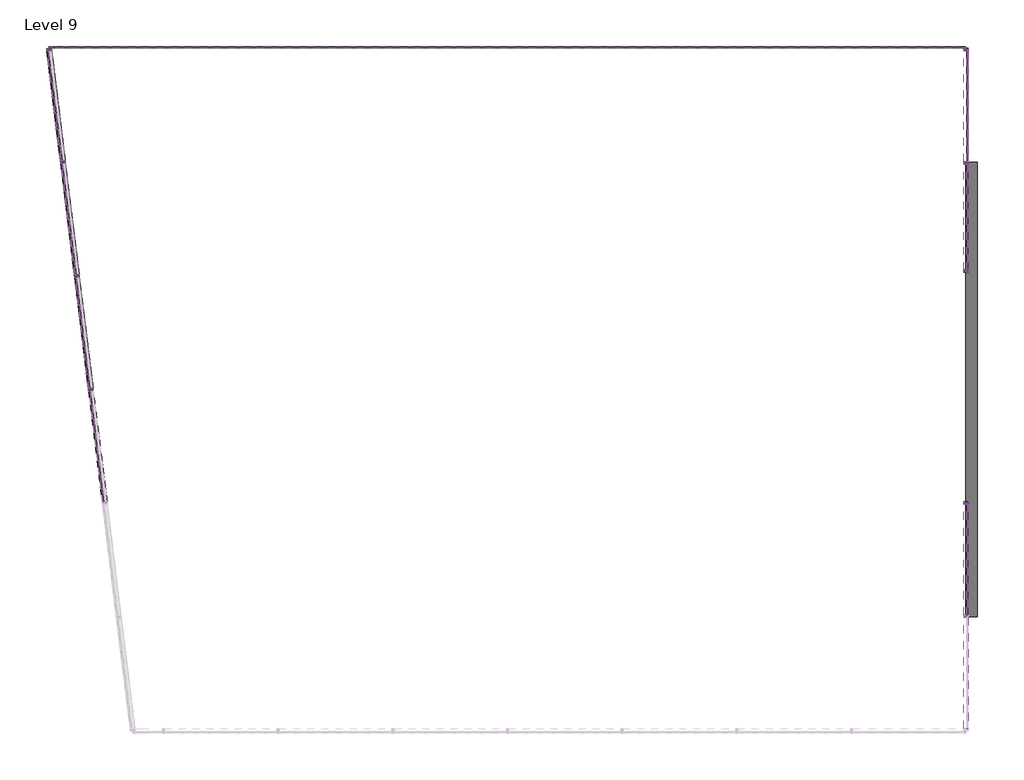
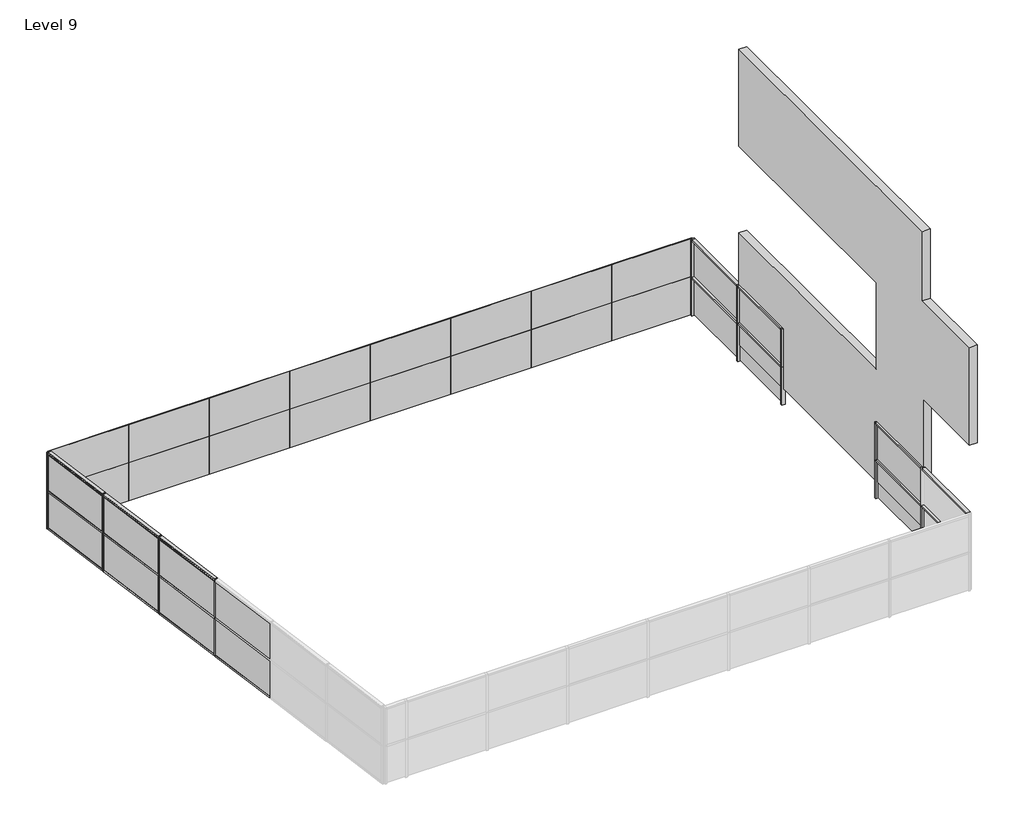
# One storey, part 2 of 2: 49 members, 38 plates, 1 proxy.
"""IFC4 building model written with IfcOpenShell, lengths in millimetres."""

from ifc_helpers import new_model, si_unit, origin, place, context, project, spatial, transform, mapped, element, save
from components import generic_models_4_generic_models_1_d225a6a7, member_71c27fd2, member_daa7a266, member_82905deb, member_19d0a4ec, member_8cef0660, member_db480205, member_4491d118, member_46bdb8c2, member_1b94d493, system_panel_glazed_1e57f9bb, system_panel_glazed_37f15d2e, system_panel_glazed_3620f98e, system_panel_glazed_e46d4b42, system_panel_glazed_2a6c68b7, system_panel_glazed_7fb1fc2b, system_panel_glazed_d483336f

model = new_model("IFC4")

# Units and contexts
model_context = context("Model", 3, world=origin())
ifc_project = project(units=[si_unit("LENGTHUNIT", "METRE", prefix="MILLI")], contexts=[model_context])

# Site, building, storey
site = spatial("IfcSite", under=ifc_project)
building = spatial("IfcBuilding", under=site)
storey = spatial("IfcBuildingStorey", under=building, Name="Level 9", Elevation=24384.0)

# Proxy
placement = place(None, origin())
generic_models_4_generic_models_1_shape = generic_models_4_generic_models_1_d225a6a7(model_context)
element("IfcBuildingElementProxy", 1, Name="Generic Models 4 : Generic Models 1", ObjectType="Generic Models 4 : Generic Models 1", at=placement, inside=storey, context=model_context, shape_type="MappedRepresentation", body=[
    mapped(generic_models_4_generic_models_1_shape, transform((0.0, 0.0, 27943.2641305), x_axis=(1.0, 0.0, 0.0), y_axis=(0.0, 1.0, 0.0), z_axis=(0.0, 0.0, 1.0))),
])

# Members
member_shape = member_71c27fd2(model_context)
element("IfcMember", 2, ObjectType="Rectangular Mullion : 2.5\" x 5\" rectangular", at=placement, inside=storey, context=model_context, shape_type="MappedRepresentation", body=[
    mapped(member_shape, transform((-10473.7456604, 11109.5209701, 24384.0), x_axis=(0.0, 0.0, -1.0), y_axis=(-0.9925461516413222, -0.12186934340514603, 0.0), z_axis=(-0.12186934340514603, 0.9925461516413222, 0.0))),
])
member_2_shape = member_daa7a266(model_context)
element("IfcMember", 3, ObjectType="Rectangular Mullion : 2.5\" x 5\" rectangular", at=placement, inside=storey, context=model_context, shape_type="MappedRepresentation", body=[
    mapped(member_2_shape, transform((-10113.8959567, 8178.7803212, 27432.0), x_axis=(0.0, 0.0, 1.0), y_axis=(-0.9925461516413222, -0.12186934340514613, 0.0), z_axis=(0.12186934340514613, -0.9925461516413222, 0.0))),
])
element("IfcMember", 4, ObjectType="Rectangular Mullion : 2.5\" x 5\" rectangular", at=placement, inside=storey, context=model_context, shape_type="MappedRepresentation", body=[
    mapped(member_2_shape, transform((13902.5156363, -946.6363705, 27432.0), x_axis=(0.0, 0.0, 1.0), y_axis=(1.0, 0.0, 0.0), z_axis=(0.0, 1.0, 0.0))),
])
element("IfcMember", 5, ObjectType="Rectangular Mullion : 2.5\" x 5\" rectangular", at=placement, inside=storey, context=model_context, shape_type="MappedRepresentation", body=[
    mapped(member_2_shape, transform((13902.5156363, -3962.8863708, 27432.0), x_axis=(0.0, 0.0, 1.0), y_axis=(1.0, 0.0, 0.0), z_axis=(0.0, 1.0, 0.0))),
])
element("IfcMember", 6, ObjectType="Rectangular Mullion : 2.5\" x 5\" rectangular", at=placement, inside=storey, context=model_context, shape_type="MappedRepresentation", body=[
    mapped(member_2_shape, transform((13902.5156363, 11109.0476508, 27432.0), x_axis=(0.0, 0.0, 1.0), y_axis=(1.0, 0.0, 0.0), z_axis=(0.0, 1.0, 0.0))),
])
member_3_shape = member_82905deb(model_context)
element("IfcMember", 7, ObjectType="Rectangular Mullion : 2.5\" x 5\" rectangular", at=placement, inside=storey, context=model_context, shape_type="MappedRepresentation", body=[
    mapped(member_3_shape, transform((-9367.1110876, 2096.7056405, 27432.0), x_axis=(-0.1218693434051459, 0.9925461516413222, 0.0), y_axis=(-0.9925461516413222, -0.1218693434051459, 0.0), z_axis=(0.0, 0.0, 1.0))),
])
element("IfcMember", 8, ObjectType="Rectangular Mullion : 2.5\" x 5\" rectangular", at=placement, inside=storey, context=model_context, shape_type="MappedRepresentation", body=[
    mapped(member_3_shape, transform((-9738.5688463, 5121.9863107, 27432.0), x_axis=(-0.1218693434051459, 0.9925461516413222, 0.0), y_axis=(-0.9925461516413222, -0.1218693434051459, 0.0), z_axis=(0.0, 0.0, 1.0))),
])
element("IfcMember", 9, ObjectType="Rectangular Mullion : 2.5\" x 5\" rectangular", at=placement, inside=storey, context=model_context, shape_type="MappedRepresentation", body=[
    mapped(member_3_shape, transform((-10110.026605, 8147.2669809, 27432.0), x_axis=(-0.1218693434051459, 0.9925461516413222, 0.0), y_axis=(-0.9925461516413222, -0.1218693434051459, 0.0), z_axis=(0.0, 0.0, 1.0))),
])
element("IfcMember", 10, ObjectType="Rectangular Mullion : 2.5\" x 5\" rectangular", at=placement, inside=storey, context=model_context, shape_type="MappedRepresentation", body=[
    mapped(member_3_shape, transform((13902.5156363, 8124.5476505, 27432.0), x_axis=(0.0, -1.0, 0.0), y_axis=(1.0, 0.0, 0.0), z_axis=(0.0, 0.0, 1.0))),
])
member_4_shape = member_19d0a4ec(model_context)
element("IfcMember", 11, ObjectType="Rectangular Mullion : 2.5\" x 5\" rectangular", at=placement, inside=storey, context=model_context, shape_type="MappedRepresentation", body=[
    mapped(member_4_shape, transform((-10113.8959567, 8178.7803212, 25908.0), x_axis=(0.0, 0.0, 1.0), y_axis=(-0.9925461516413222, -0.12186934340514603, 0.0), z_axis=(0.12186934340514603, -0.9925461516413222, 0.0))),
])
element("IfcMember", 12, ObjectType="Rectangular Mullion : 2.5\" x 5\" rectangular", at=placement, inside=storey, context=model_context, shape_type="MappedRepresentation", body=[
    mapped(member_4_shape, transform((-10113.8959567, 8178.7803212, 27432.0), x_axis=(0.0, 0.0, 1.0), y_axis=(-0.9925461516413223, -0.12186934340514535, 0.0), z_axis=(0.12186934340514535, -0.9925461516413223, 0.0))),
])
element("IfcMember", 13, ObjectType="Rectangular Mullion : 2.5\" x 5\" rectangular", at=placement, inside=storey, context=model_context, shape_type="MappedRepresentation", body=[
    mapped(member_4_shape, transform((-10113.8959567, 8178.7803212, 25908.0), x_axis=(0.0, 0.0, 1.0), y_axis=(-0.9925461516413222, -0.12186934340514599, 0.0), z_axis=(0.12186934340514599, -0.9925461516413222, 0.0))),
])
element("IfcMember", 14, ObjectType="Rectangular Mullion : 2.5\" x 5\" rectangular", at=placement, inside=storey, context=model_context, shape_type="MappedRepresentation", body=[
    mapped(member_4_shape, transform((13902.5156363, -946.6363705, 25908.0), x_axis=(0.0, 0.0, 1.0), y_axis=(1.0, 0.0, 0.0), z_axis=(0.0, 1.0, 0.0))),
])
element("IfcMember", 15, ObjectType="Rectangular Mullion : 2.5\" x 5\" rectangular", at=placement, inside=storey, context=model_context, shape_type="MappedRepresentation", body=[
    mapped(member_4_shape, transform((13902.5156363, -3962.8863708, 25908.0), x_axis=(0.0, 0.0, 1.0), y_axis=(1.0, 0.0, 0.0), z_axis=(0.0, 1.0, 0.0))),
])
element("IfcMember", 16, ObjectType="Rectangular Mullion : 2.5\" x 5\" rectangular", at=placement, inside=storey, context=model_context, shape_type="MappedRepresentation", body=[
    mapped(member_4_shape, transform((13902.5156363, 11109.0476508, 25908.0), x_axis=(0.0, 0.0, 1.0), y_axis=(1.0, 0.0, 0.0), z_axis=(0.0, 1.0, 0.0))),
])
member_5_shape = member_8cef0660(model_context)
element("IfcMember", 17, ObjectType="Rectangular Mullion : 2.5\" x 5\" rectangular", at=placement, inside=storey, context=model_context, shape_type="MappedRepresentation", body=[
    mapped(member_5_shape, transform((-9370.9804393, 2128.2189808, 25908.0), x_axis=(0.0, 0.0, 1.0), y_axis=(-0.9925461516413222, -0.12186934340514592, 0.0), z_axis=(0.12186934340514592, -0.9925461516413222, 0.0))),
])
element("IfcMember", 18, ObjectType="Rectangular Mullion : 2.5\" x 5\" rectangular", at=placement, inside=storey, context=model_context, shape_type="MappedRepresentation", body=[
    mapped(member_5_shape, transform((-9742.438198, 5153.499651, 25908.0), x_axis=(0.0, 0.0, 1.0), y_axis=(-0.9925461516413222, -0.12186934340514574, 0.0), z_axis=(0.12186934340514574, -0.9925461516413222, 0.0))),
])
element("IfcMember", 19, ObjectType="Rectangular Mullion : 2.5\" x 5\" rectangular", at=placement, inside=storey, context=model_context, shape_type="MappedRepresentation", body=[
    mapped(member_5_shape, transform((-9370.9804393, 2128.2189808, 27432.0), x_axis=(0.0, 0.0, 1.0), y_axis=(-0.9925461516413222, -0.12186934340514592, 0.0), z_axis=(0.12186934340514592, -0.9925461516413222, 0.0))),
])
element("IfcMember", 20, ObjectType="Rectangular Mullion : 2.5\" x 5\" rectangular", at=placement, inside=storey, context=model_context, shape_type="MappedRepresentation", body=[
    mapped(member_5_shape, transform((-9742.438198, 5153.499651, 27432.0), x_axis=(0.0, 0.0, 1.0), y_axis=(-0.9925461516413222, -0.1218693434051461, 0.0), z_axis=(0.1218693434051461, -0.9925461516413222, 0.0))),
])
element("IfcMember", 21, ObjectType="Rectangular Mullion : 2.5\" x 5\" rectangular", at=placement, inside=storey, context=model_context, shape_type="MappedRepresentation", body=[
    mapped(member_5_shape, transform((-9370.9804393, 2128.2189808, 25908.0), x_axis=(0.0, 0.0, 1.0), y_axis=(-0.9925461516413222, -0.12186934340514596, 0.0), z_axis=(0.12186934340514596, -0.9925461516413222, 0.0))),
])
element("IfcMember", 22, ObjectType="Rectangular Mullion : 2.5\" x 5\" rectangular", at=placement, inside=storey, context=model_context, shape_type="MappedRepresentation", body=[
    mapped(member_5_shape, transform((-9742.438198, 5153.499651, 25908.0), x_axis=(0.0, 0.0, 1.0), y_axis=(-0.9925461516413222, -0.12186934340514606, 0.0), z_axis=(0.12186934340514606, -0.9925461516413222, 0.0))),
])
member_6_shape = member_db480205(model_context)
element("IfcMember", 23, ObjectType="Rectangular Mullion : 2.5\" x 5\" rectangular", at=placement, inside=storey, context=model_context, shape_type="MappedRepresentation", body=[
    mapped(member_6_shape, transform((-9363.241736, 2065.1923001, 24384.0), x_axis=(0.0, 0.0, -1.0), y_axis=(-0.9925461516413222, -0.12186934340514602, 0.0), z_axis=(-0.12186934340514602, 0.9925461516413222, 0.0))),
])
element("IfcMember", 24, ObjectType="Rectangular Mullion : 2.5\" x 5\" rectangular", at=placement, inside=storey, context=model_context, shape_type="MappedRepresentation", body=[
    mapped(member_6_shape, transform((-9734.6994947, 5090.4729703, 24384.0), x_axis=(0.0, 0.0, -1.0), y_axis=(-0.9925461516413223, -0.12186934340514559, 0.0), z_axis=(-0.12186934340514559, 0.9925461516413223, 0.0))),
])
element("IfcMember", 25, ObjectType="Rectangular Mullion : 2.5\" x 5\" rectangular", at=placement, inside=storey, context=model_context, shape_type="MappedRepresentation", body=[
    mapped(member_6_shape, transform((-10106.1572534, 8115.7536405, 24384.0), x_axis=(0.0, 0.0, -1.0), y_axis=(-0.9925461516413222, -0.1218693434051461, 0.0), z_axis=(-0.1218693434051461, 0.9925461516413222, 0.0))),
])
element("IfcMember", 26, ObjectType="Rectangular Mullion : 2.5\" x 5\" rectangular", at=placement, inside=storey, context=model_context, shape_type="MappedRepresentation", body=[
    mapped(member_6_shape, transform((-9370.9804393, 2128.2189808, 27432.0), x_axis=(0.0, 0.0, 1.0), y_axis=(-0.9925461516413223, -0.12186934340514563, 0.0), z_axis=(0.12186934340514562, -0.9925461516413222, 0.0))),
])
element("IfcMember", 27, ObjectType="Rectangular Mullion : 2.5\" x 5\" rectangular", at=placement, inside=storey, context=model_context, shape_type="MappedRepresentation", body=[
    mapped(member_6_shape, transform((-9742.438198, 5153.499651, 27432.0), x_axis=(0.0, 0.0, 1.0), y_axis=(-0.9925461516413222, -0.1218693434051461, 0.0), z_axis=(0.1218693434051461, -0.9925461516413222, 0.0))),
])
element("IfcMember", 28, ObjectType="Rectangular Mullion : 2.5\" x 5\" rectangular", at=placement, inside=storey, context=model_context, shape_type="MappedRepresentation", body=[
    mapped(member_3_shape, transform((-9367.1110876, 2096.7056405, 25908.0), x_axis=(-0.1218693434051459, 0.9925461516413222, 0.0), y_axis=(-0.9925461516413222, -0.1218693434051459, 0.0), z_axis=(0.0, 0.0, 1.0))),
])
element("IfcMember", 29, ObjectType="Rectangular Mullion : 2.5\" x 5\" rectangular", at=placement, inside=storey, context=model_context, shape_type="MappedRepresentation", body=[
    mapped(member_3_shape, transform((-9738.5688463, 5121.9863107, 25908.0), x_axis=(-0.1218693434051459, 0.9925461516413222, 0.0), y_axis=(-0.9925461516413222, -0.1218693434051459, 0.0), z_axis=(0.0, 0.0, 1.0))),
])
element("IfcMember", 30, ObjectType="Rectangular Mullion : 2.5\" x 5\" rectangular", at=placement, inside=storey, context=model_context, shape_type="MappedRepresentation", body=[
    mapped(member_3_shape, transform((-10110.026605, 8147.2669809, 25908.0), x_axis=(-0.1218693434051459, 0.9925461516413222, 0.0), y_axis=(-0.9925461516413222, -0.1218693434051459, 0.0), z_axis=(0.0, 0.0, 1.0))),
])
element("IfcMember", 31, ObjectType="Rectangular Mullion : 2.5\" x 5\" rectangular", at=placement, inside=storey, context=model_context, shape_type="MappedRepresentation", body=[
    mapped(member_3_shape, transform((-9367.1110876, 2096.7056405, 27432.0), x_axis=(-0.1218693434051459, 0.9925461516413222, 0.0), y_axis=(-0.9925461516413222, -0.1218693434051459, 0.0), z_axis=(0.0, 0.0, 1.0))),
])
element("IfcMember", 32, ObjectType="Rectangular Mullion : 2.5\" x 5\" rectangular", at=placement, inside=storey, context=model_context, shape_type="MappedRepresentation", body=[
    mapped(member_3_shape, transform((-9738.5688463, 5121.9863107, 27432.0), x_axis=(-0.1218693434051459, 0.9925461516413222, 0.0), y_axis=(-0.9925461516413222, -0.1218693434051459, 0.0), z_axis=(0.0, 0.0, 1.0))),
])
element("IfcMember", 33, ObjectType="Rectangular Mullion : 2.5\" x 5\" rectangular", at=placement, inside=storey, context=model_context, shape_type="MappedRepresentation", body=[
    mapped(member_3_shape, transform((-10110.026605, 8147.2669809, 27432.0), x_axis=(-0.1218693434051459, 0.9925461516413222, 0.0), y_axis=(-0.9925461516413222, -0.1218693434051459, 0.0), z_axis=(0.0, 0.0, 1.0))),
])
element("IfcMember", 34, ObjectType="Rectangular Mullion : 2.5\" x 5\" rectangular", at=placement, inside=storey, context=model_context, shape_type="MappedRepresentation", body=[
    mapped(member_3_shape, transform((-9367.1110876, 2096.7056405, 25908.0), x_axis=(-0.1218693434051459, 0.9925461516413222, 0.0), y_axis=(-0.9925461516413222, -0.1218693434051459, 0.0), z_axis=(0.0, 0.0, 1.0))),
])
element("IfcMember", 35, ObjectType="Rectangular Mullion : 2.5\" x 5\" rectangular", at=placement, inside=storey, context=model_context, shape_type="MappedRepresentation", body=[
    mapped(member_3_shape, transform((-9738.5688463, 5121.9863107, 25908.0), x_axis=(-0.1218693434051459, 0.9925461516413222, 0.0), y_axis=(-0.9925461516413222, -0.1218693434051459, 0.0), z_axis=(0.0, 0.0, 1.0))),
])
element("IfcMember", 36, ObjectType="Rectangular Mullion : 2.5\" x 5\" rectangular", at=placement, inside=storey, context=model_context, shape_type="MappedRepresentation", body=[
    mapped(member_3_shape, transform((-10110.026605, 8147.2669809, 25908.0), x_axis=(-0.1218693434051459, 0.9925461516413222, 0.0), y_axis=(-0.9925461516413222, -0.1218693434051459, 0.0), z_axis=(0.0, 0.0, 1.0))),
])
element("IfcMember", 37, ObjectType="Rectangular Mullion : 2.5\" x 5\" rectangular", at=placement, inside=storey, context=model_context, shape_type="MappedRepresentation", body=[
    mapped(member_3_shape, transform((13902.5156363, -3931.1363708, 25908.0), x_axis=(0.0, -1.0, 0.0), y_axis=(1.0, 0.0, 0.0), z_axis=(0.0, 0.0, 1.0))),
])
element("IfcMember", 38, ObjectType="Rectangular Mullion : 2.5\" x 5\" rectangular", at=placement, inside=storey, context=model_context, shape_type="MappedRepresentation", body=[
    mapped(member_3_shape, transform((13902.5156363, 8124.5476505, 25908.0), x_axis=(0.0, -1.0, 0.0), y_axis=(1.0, 0.0, 0.0), z_axis=(0.0, 0.0, 1.0))),
])
member_7_shape = member_4491d118(model_context)
element("IfcMember", 39, ObjectType="Rectangular Mullion : 2.5\" x 5\" rectangular", at=placement, inside=storey, context=model_context, shape_type="MappedRepresentation", body=[
    mapped(member_7_shape, transform((-10481.4843637, 11172.5476508, 27432.0), x_axis=(-0.1218693434051459, 0.9925461516413222, 0.0), y_axis=(-0.9925461516413222, -0.1218693434051459, 0.0), z_axis=(0.0, 0.0, 1.0))),
])
element("IfcMember", 40, ObjectType="Rectangular Mullion : 2.5\" x 5\" rectangular", at=placement, inside=storey, context=model_context, shape_type="MappedRepresentation", body=[
    mapped(member_7_shape, transform((13902.5156363, 5212.8636295, 27432.0), x_axis=(0.0, -1.0, 0.0), y_axis=(1.0, 0.0, 0.0), z_axis=(0.0, 0.0, 1.0))),
])
element("IfcMember", 41, ObjectType="Rectangular Mullion : 2.5\" x 5\" rectangular", at=placement, inside=storey, context=model_context, shape_type="MappedRepresentation", body=[
    mapped(member_7_shape, transform((13902.5156363, -883.1363705, 24384.0), x_axis=(0.0, 1.0, 0.0), y_axis=(1.0, 0.0, 0.0), z_axis=(0.0, 0.0, -1.0))),
])
element("IfcMember", 42, ObjectType="Rectangular Mullion : 2.5\" x 5\" rectangular", at=placement, inside=storey, context=model_context, shape_type="MappedRepresentation", body=[
    mapped(member_7_shape, transform((13902.5156363, 11172.5476508, 24384.0), x_axis=(0.0, 1.0, 0.0), y_axis=(1.0, 0.0, 0.0), z_axis=(0.0, 0.0, -1.0))),
])
element("IfcMember", 43, ObjectType="Rectangular Mullion : 2.5\" x 5\" rectangular", at=placement, inside=storey, context=model_context, shape_type="MappedRepresentation", body=[
    mapped(member_7_shape, transform((13902.5156363, -883.1363705, 25908.0), x_axis=(0.0, 1.0, 0.0), y_axis=(1.0, 0.0, 0.0), z_axis=(0.0, 0.0, -1.0))),
])
element("IfcMember", 44, ObjectType="Rectangular Mullion : 2.5\" x 5\" rectangular", at=placement, inside=storey, context=model_context, shape_type="MappedRepresentation", body=[
    mapped(member_7_shape, transform((13902.5156363, 11172.5476508, 25908.0), x_axis=(0.0, 1.0, 0.0), y_axis=(1.0, 0.0, 0.0), z_axis=(0.0, 0.0, -1.0))),
])
element("IfcMember", 45, ObjectType="Rectangular Mullion : 2.5\" x 5\" rectangular", at=placement, inside=storey, context=model_context, shape_type="MappedRepresentation", body=[
    mapped(member_7_shape, transform((-10481.4843637, 11172.5476508, 25908.0), x_axis=(-0.1218693434051459, 0.9925461516413222, 0.0), y_axis=(-0.9925461516413222, -0.1218693434051459, 0.0), z_axis=(0.0, 0.0, 1.0))),
])
element("IfcMember", 46, ObjectType="Rectangular Mullion : 2.5\" x 5\" rectangular", at=placement, inside=storey, context=model_context, shape_type="MappedRepresentation", body=[
    mapped(member_7_shape, transform((-10481.4843637, 11172.5476508, 27432.0), x_axis=(-0.1218693434051459, 0.9925461516413222, 0.0), y_axis=(-0.9925461516413222, -0.1218693434051459, 0.0), z_axis=(0.0, 0.0, 1.0))),
])
element("IfcMember", 47, ObjectType="Rectangular Mullion : 2.5\" x 5\" rectangular", at=placement, inside=storey, context=model_context, shape_type="MappedRepresentation", body=[
    mapped(member_7_shape, transform((-10481.4843637, 11172.5476508, 25908.0), x_axis=(-0.1218693434051459, 0.9925461516413222, 0.0), y_axis=(-0.9925461516413222, -0.1218693434051459, 0.0), z_axis=(0.0, 0.0, 1.0))),
])
element("IfcMember", 48, ObjectType="Rectangular Mullion : 2.5\" x 5\" rectangular", at=placement, inside=storey, context=model_context, shape_type="MappedRepresentation", body=[
    mapped(member_7_shape, transform((13902.5156363, 5212.8636295, 25908.0), x_axis=(0.0, -1.0, 0.0), y_axis=(1.0, 0.0, 0.0), z_axis=(0.0, 0.0, 1.0))),
])
member_8_shape = member_46bdb8c2(model_context)
element("IfcMember", 49, ObjectType="Rectangular Mullion : 2.5\" x 5\" rectangular", at=placement, inside=storey, context=model_context, shape_type="MappedRepresentation", body=[
    mapped(member_8_shape, transform((13902.5156363, 8092.7976505, 25908.0), x_axis=(0.0, 0.0, 1.0), y_axis=(1.0, 0.0, 0.0), z_axis=(0.0, 1.0, 0.0))),
])
member_9_shape = member_1b94d493(model_context)
element("IfcMember", 50, ObjectType="Rectangular Mullion : 2.5\" x 5\" rectangular", at=placement, inside=storey, context=model_context, shape_type="MappedRepresentation", body=[
    mapped(member_9_shape, transform((13902.5156363, 8092.7976505, 27432.0), x_axis=(0.0, 0.0, 1.0), y_axis=(1.0, 0.0, 0.0), z_axis=(0.0, 1.0, 0.0))),
])

# Plates
system_panel_glazed_shape = system_panel_glazed_1e57f9bb(model_context)
element("IfcPlate", 51, ObjectType="System Panel : Glazed", at=placement, inside=storey, context=model_context, shape_type="MappedRepresentation", body=[
    mapped(system_panel_glazed_shape, transform((-8957.4843636, 11172.5476508, 24384.0), x_axis=(1.0, 0.0, 0.0), y_axis=(0.0, 1.0, 0.0), z_axis=(0.0, 0.0, 1.0))),
])
element("IfcPlate", 52, ObjectType="System Panel : Glazed", at=placement, inside=storey, context=model_context, shape_type="MappedRepresentation", body=[
    mapped(system_panel_glazed_shape, transform((-5909.4843634, 11172.5476508, 24384.0), x_axis=(1.0, 0.0, 0.0), y_axis=(0.0, 1.0, 0.0), z_axis=(0.0, 0.0, 1.0))),
])
element("IfcPlate", 53, ObjectType="System Panel : Glazed", at=placement, inside=storey, context=model_context, shape_type="MappedRepresentation", body=[
    mapped(system_panel_glazed_shape, transform((-2861.4843634, 11172.5476508, 24384.0), x_axis=(1.0, 0.0, 0.0), y_axis=(0.0, 1.0, 0.0), z_axis=(0.0, 0.0, 1.0))),
])
element("IfcPlate", 54, ObjectType="System Panel : Glazed", at=placement, inside=storey, context=model_context, shape_type="MappedRepresentation", body=[
    mapped(system_panel_glazed_shape, transform((186.5156366, 11172.5476508, 24384.0), x_axis=(1.0, 0.0, 0.0), y_axis=(0.0, 1.0, 0.0), z_axis=(0.0, 0.0, 1.0))),
])
element("IfcPlate", 55, ObjectType="System Panel : Glazed", at=placement, inside=storey, context=model_context, shape_type="MappedRepresentation", body=[
    mapped(system_panel_glazed_shape, transform((3234.5156366, 11172.5476508, 24384.0), x_axis=(1.0, 0.0, 0.0), y_axis=(0.0, 1.0, 0.0), z_axis=(0.0, 0.0, 1.0))),
])
element("IfcPlate", 56, ObjectType="System Panel : Glazed", at=placement, inside=storey, context=model_context, shape_type="MappedRepresentation", body=[
    mapped(system_panel_glazed_shape, transform((6282.5156366, 11172.5476508, 24384.0), x_axis=(1.0, 0.0, 0.0), y_axis=(0.0, 1.0, 0.0), z_axis=(0.0, 0.0, 1.0))),
])
element("IfcPlate", 57, ObjectType="System Panel : Glazed", at=placement, inside=storey, context=model_context, shape_type="MappedRepresentation", body=[
    mapped(system_panel_glazed_shape, transform((9330.5156366, 11172.5476508, 24384.0), x_axis=(1.0, 0.0, 0.0), y_axis=(0.0, 1.0, 0.0), z_axis=(0.0, 0.0, 1.0))),
])
element("IfcPlate", 58, ObjectType="System Panel : Glazed", at=placement, inside=storey, context=model_context, shape_type="MappedRepresentation", body=[
    mapped(system_panel_glazed_shape, transform((12378.5156364, 11172.5476508, 24384.0), x_axis=(1.0, 0.0, 0.0), y_axis=(0.0, 1.0, 0.0), z_axis=(0.0, 0.0, 1.0))),
])
element("IfcPlate", 59, ObjectType="System Panel : Glazed", at=placement, inside=storey, context=model_context, shape_type="MappedRepresentation", body=[
    mapped(system_panel_glazed_shape, transform((-8957.4843636, 11172.5476508, 25908.0), x_axis=(1.0, 0.0, 0.0), y_axis=(0.0, 1.0, 0.0), z_axis=(0.0, 0.0, 1.0))),
])
element("IfcPlate", 60, ObjectType="System Panel : Glazed", at=placement, inside=storey, context=model_context, shape_type="MappedRepresentation", body=[
    mapped(system_panel_glazed_shape, transform((-5909.4843634, 11172.5476508, 25908.0), x_axis=(1.0, 0.0, 0.0), y_axis=(0.0, 1.0, 0.0), z_axis=(0.0, 0.0, 1.0))),
])
element("IfcPlate", 61, ObjectType="System Panel : Glazed", at=placement, inside=storey, context=model_context, shape_type="MappedRepresentation", body=[
    mapped(system_panel_glazed_shape, transform((-2861.4843634, 11172.5476508, 25908.0), x_axis=(1.0, 0.0, 0.0), y_axis=(0.0, 1.0, 0.0), z_axis=(0.0, 0.0, 1.0))),
])
element("IfcPlate", 62, ObjectType="System Panel : Glazed", at=placement, inside=storey, context=model_context, shape_type="MappedRepresentation", body=[
    mapped(system_panel_glazed_shape, transform((186.5156366, 11172.5476508, 25908.0), x_axis=(1.0, 0.0, 0.0), y_axis=(0.0, 1.0, 0.0), z_axis=(0.0, 0.0, 1.0))),
])
element("IfcPlate", 63, ObjectType="System Panel : Glazed", at=placement, inside=storey, context=model_context, shape_type="MappedRepresentation", body=[
    mapped(system_panel_glazed_shape, transform((3234.5156366, 11172.5476508, 25908.0), x_axis=(1.0, 0.0, 0.0), y_axis=(0.0, 1.0, 0.0), z_axis=(0.0, 0.0, 1.0))),
])
element("IfcPlate", 64, ObjectType="System Panel : Glazed", at=placement, inside=storey, context=model_context, shape_type="MappedRepresentation", body=[
    mapped(system_panel_glazed_shape, transform((6282.5156366, 11172.5476508, 25908.0), x_axis=(1.0, 0.0, 0.0), y_axis=(0.0, 1.0, 0.0), z_axis=(0.0, 0.0, 1.0))),
])
element("IfcPlate", 65, ObjectType="System Panel : Glazed", at=placement, inside=storey, context=model_context, shape_type="MappedRepresentation", body=[
    mapped(system_panel_glazed_shape, transform((9330.5156366, 11172.5476508, 25908.0), x_axis=(1.0, 0.0, 0.0), y_axis=(0.0, 1.0, 0.0), z_axis=(0.0, 0.0, 1.0))),
])
element("IfcPlate", 66, ObjectType="System Panel : Glazed", at=placement, inside=storey, context=model_context, shape_type="MappedRepresentation", body=[
    mapped(system_panel_glazed_shape, transform((12378.5156364, 11172.5476508, 25908.0), x_axis=(1.0, 0.0, 0.0), y_axis=(0.0, 1.0, 0.0), z_axis=(0.0, 0.0, 1.0))),
])
system_panel_glazed_2_shape = system_panel_glazed_37f15d2e(model_context)
element("IfcPlate", 67, ObjectType="System Panel : Glazed", at=placement, inside=storey, context=model_context, shape_type="MappedRepresentation", body=[
    mapped(system_panel_glazed_2_shape, transform((-10293.8208085, 9644.1506457, 25939.75), x_axis=(-0.1218693434051459, 0.9925461516413222, 0.0), y_axis=(-0.9925461516413222, -0.1218693434051459, 0.0), z_axis=(0.0, 0.0, 1.0))),
])
element("IfcPlate", 68, ObjectType="System Panel : Glazed", at=placement, inside=storey, context=model_context, shape_type="MappedRepresentation", body=[
    mapped(system_panel_glazed_2_shape, transform((13902.5156363, -2423.0113706, 25939.75), x_axis=(0.0, -1.0, 0.0), y_axis=(1.0, 0.0, 0.0), z_axis=(0.0, 0.0, 1.0))),
])
element("IfcPlate", 69, ObjectType="System Panel : Glazed", at=placement, inside=storey, context=model_context, shape_type="MappedRepresentation", body=[
    mapped(system_panel_glazed_2_shape, transform((13902.5156363, 9632.6726506, 25939.75), x_axis=(0.0, -1.0, 0.0), y_axis=(1.0, 0.0, 0.0), z_axis=(0.0, 0.0, 1.0))),
])
element("IfcPlate", 70, ObjectType="System Panel : Glazed", at=placement, inside=storey, context=model_context, shape_type="MappedRepresentation", body=[
    mapped(system_panel_glazed_2_shape, transform((-10293.8208085, 9644.1506457, 24447.5), x_axis=(-0.1218693434051459, 0.9925461516413222, 0.0), y_axis=(-0.9925461516413222, -0.1218693434051459, 0.0), z_axis=(0.0, 0.0, 1.0))),
])
system_panel_glazed_3_shape = system_panel_glazed_3620f98e(model_context)
element("IfcPlate", 71, ObjectType="System Panel : Glazed", at=placement, inside=storey, context=model_context, shape_type="MappedRepresentation", body=[
    mapped(system_panel_glazed_3_shape, transform((-9181.3822083, 584.0653054, 25939.75), x_axis=(-0.1218693434051459, 0.9925461516413222, 0.0), y_axis=(-0.9925461516413222, -0.1218693434051459, 0.0), z_axis=(0.0, 0.0, 1.0))),
])
element("IfcPlate", 72, ObjectType="System Panel : Glazed", at=placement, inside=storey, context=model_context, shape_type="MappedRepresentation", body=[
    mapped(system_panel_glazed_3_shape, transform((-9552.839967, 3609.3459756, 25939.75), x_axis=(-0.1218693434051459, 0.9925461516413222, 0.0), y_axis=(-0.9925461516413222, -0.1218693434051459, 0.0), z_axis=(0.0, 0.0, 1.0))),
])
element("IfcPlate", 73, ObjectType="System Panel : Glazed", at=placement, inside=storey, context=model_context, shape_type="MappedRepresentation", body=[
    mapped(system_panel_glazed_3_shape, transform((-9924.2977257, 6634.6266458, 25939.75), x_axis=(-0.1218693434051459, 0.9925461516413222, 0.0), y_axis=(-0.9925461516413222, -0.1218693434051459, 0.0), z_axis=(0.0, 0.0, 1.0))),
])
element("IfcPlate", 74, ObjectType="System Panel : Glazed", at=placement, inside=storey, context=model_context, shape_type="MappedRepresentation", body=[
    mapped(system_panel_glazed_3_shape, transform((-9181.3822083, 584.0653054, 24447.5), x_axis=(-0.1218693434051459, 0.9925461516413222, 0.0), y_axis=(-0.9925461516413222, -0.1218693434051459, 0.0), z_axis=(0.0, 0.0, 1.0))),
])
element("IfcPlate", 75, ObjectType="System Panel : Glazed", at=placement, inside=storey, context=model_context, shape_type="MappedRepresentation", body=[
    mapped(system_panel_glazed_3_shape, transform((-9552.839967, 3609.3459756, 24447.5), x_axis=(-0.1218693434051459, 0.9925461516413222, 0.0), y_axis=(-0.9925461516413222, -0.1218693434051459, 0.0), z_axis=(0.0, 0.0, 1.0))),
])
element("IfcPlate", 76, ObjectType="System Panel : Glazed", at=placement, inside=storey, context=model_context, shape_type="MappedRepresentation", body=[
    mapped(system_panel_glazed_3_shape, transform((-9924.2977257, 6634.6266458, 24447.5), x_axis=(-0.1218693434051459, 0.9925461516413222, 0.0), y_axis=(-0.9925461516413222, -0.1218693434051459, 0.0), z_axis=(0.0, 0.0, 1.0))),
])
system_panel_glazed_4_shape = system_panel_glazed_e46d4b42(model_context)
element("IfcPlate", 77, ObjectType="System Panel : Glazed", at=placement, inside=storey, context=model_context, shape_type="MappedRepresentation", body=[
    mapped(system_panel_glazed_4_shape, transform((-10293.8208085, 9644.1506457, 24415.75), x_axis=(-0.1218693434051459, 0.9925461516413222, 0.0), y_axis=(-0.9925461516413222, -0.1218693434051459, 0.0), z_axis=(0.0, 0.0, 1.0))),
])
element("IfcPlate", 78, ObjectType="System Panel : Glazed", at=placement, inside=storey, context=model_context, shape_type="MappedRepresentation", body=[
    mapped(system_panel_glazed_4_shape, transform((13902.5156363, -2423.0113706, 24415.75), x_axis=(0.0, -1.0, 0.0), y_axis=(1.0, 0.0, 0.0), z_axis=(0.0, 0.0, 1.0))),
])
element("IfcPlate", 79, ObjectType="System Panel : Glazed", at=placement, inside=storey, context=model_context, shape_type="MappedRepresentation", body=[
    mapped(system_panel_glazed_4_shape, transform((13902.5156363, 9632.6726506, 24415.75), x_axis=(0.0, -1.0, 0.0), y_axis=(1.0, 0.0, 0.0), z_axis=(0.0, 0.0, 1.0))),
])
element("IfcPlate", 80, ObjectType="System Panel : Glazed", at=placement, inside=storey, context=model_context, shape_type="MappedRepresentation", body=[
    mapped(system_panel_glazed_4_shape, transform((-10293.8208085, 9644.1506457, 25939.75), x_axis=(-0.1218693434051459, 0.9925461516413222, 0.0), y_axis=(-0.9925461516413222, -0.1218693434051459, 0.0), z_axis=(0.0, 0.0, 1.0))),
])
system_panel_glazed_5_shape = system_panel_glazed_2a6c68b7(model_context)
element("IfcPlate", 81, ObjectType="System Panel : Glazed", at=placement, inside=storey, context=model_context, shape_type="MappedRepresentation", body=[
    mapped(system_panel_glazed_5_shape, transform((-9181.3822083, 584.0653054, 24415.75), x_axis=(-0.1218693434051459, 0.9925461516413222, 0.0), y_axis=(-0.9925461516413222, -0.1218693434051459, 0.0), z_axis=(0.0, 0.0, 1.0))),
])
element("IfcPlate", 82, ObjectType="System Panel : Glazed", at=placement, inside=storey, context=model_context, shape_type="MappedRepresentation", body=[
    mapped(system_panel_glazed_5_shape, transform((-9552.839967, 3609.3459756, 24415.75), x_axis=(-0.1218693434051459, 0.9925461516413222, 0.0), y_axis=(-0.9925461516413222, -0.1218693434051459, 0.0), z_axis=(0.0, 0.0, 1.0))),
])
element("IfcPlate", 83, ObjectType="System Panel : Glazed", at=placement, inside=storey, context=model_context, shape_type="MappedRepresentation", body=[
    mapped(system_panel_glazed_5_shape, transform((-9924.2977257, 6634.6266458, 24415.75), x_axis=(-0.1218693434051459, 0.9925461516413222, 0.0), y_axis=(-0.9925461516413222, -0.1218693434051459, 0.0), z_axis=(0.0, 0.0, 1.0))),
])
element("IfcPlate", 84, ObjectType="System Panel : Glazed", at=placement, inside=storey, context=model_context, shape_type="MappedRepresentation", body=[
    mapped(system_panel_glazed_5_shape, transform((-9181.3822083, 584.0653054, 25939.75), x_axis=(-0.1218693434051459, 0.9925461516413222, 0.0), y_axis=(-0.9925461516413222, -0.1218693434051459, 0.0), z_axis=(0.0, 0.0, 1.0))),
])
element("IfcPlate", 85, ObjectType="System Panel : Glazed", at=placement, inside=storey, context=model_context, shape_type="MappedRepresentation", body=[
    mapped(system_panel_glazed_5_shape, transform((-9552.839967, 3609.3459756, 25939.75), x_axis=(-0.1218693434051459, 0.9925461516413222, 0.0), y_axis=(-0.9925461516413222, -0.1218693434051459, 0.0), z_axis=(0.0, 0.0, 1.0))),
])
element("IfcPlate", 86, ObjectType="System Panel : Glazed", at=placement, inside=storey, context=model_context, shape_type="MappedRepresentation", body=[
    mapped(system_panel_glazed_5_shape, transform((-9924.2977257, 6634.6266458, 25939.75), x_axis=(-0.1218693434051459, 0.9925461516413222, 0.0), y_axis=(-0.9925461516413222, -0.1218693434051459, 0.0), z_axis=(0.0, 0.0, 1.0))),
])
system_panel_glazed_6_shape = system_panel_glazed_7fb1fc2b(model_context)
element("IfcPlate", 87, ObjectType="System Panel : Glazed", at=placement, inside=storey, context=model_context, shape_type="MappedRepresentation", body=[
    mapped(system_panel_glazed_6_shape, transform((13902.5156363, 6684.58064, 25939.75), x_axis=(0.0, -1.0, 0.0), y_axis=(1.0, 0.0, 0.0), z_axis=(0.0, 0.0, 1.0))),
])
system_panel_glazed_7_shape = system_panel_glazed_d483336f(model_context)
element("IfcPlate", 88, ObjectType="System Panel : Glazed", at=placement, inside=storey, context=model_context, shape_type="MappedRepresentation", body=[
    mapped(system_panel_glazed_7_shape, transform((13902.5156363, 6684.58064, 24415.75), x_axis=(0.0, -1.0, 0.0), y_axis=(1.0, 0.0, 0.0), z_axis=(0.0, 0.0, 1.0))),
])

save(model, "model.ifc")

# Revit data of these elements
# Type "Rectangular Mullion : 2.5\" x 5\" rectangular"
#   built-in parameter 1007304 = 0.416667 (stored number, unit not read)
#   built-in parameter 1007301 = 0.104167 (stored number, unit not read)
#   built-in parameter 1007300 = 0.104167 (stored number, unit not read)
# Type "System Panel : Glazed"
#   Construction Type Id = "GSP4R"
#   Analytic Construction = "1/8 in Pilkington single glazing"
#   Visual Light Transmittance = 0.9
#   Solar Heat Gain Coefficient = 0.86
#   Heat Transfer Coefficient (U) = 1.18115 BTU/(h·ft²·°F)
#   Define Thermal Properties by = 1
# Element 1 (IfcBuildingElementProxy, "Generic Models 4 : Generic Models 1")
#   Phase Created = New Construction
# Elements 2, 3, 4, 5, 6, 7, 8, 9, 10, 11, 12, 13, 14, 15, 16, 17, 18, 19, 20, 21, 22, 23, 24, 25, 26, 27, 28, 29, 30, 31, 32, 33, 34, 35, 36, 37, 38, 39, 40, 41, 42, 43, 44, 45, 46, 47, 48, 49, 50 (IfcMember, "Rectangular Mullion : 2.5\" x 5\" rectangular")
#   Phase Created = New Construction
#   Materials on its faces: "Aluminum"
# Elements 51, 52, 53, 54, 55, 56, 57, 58, 59, 60, 61, 62, 63, 64, 65, 66, 67, 68, 69, 70, 71, 72, 73, 74, 75, 76, 77, 78, 79, 80, 81, 82, 83, 84, 85, 86, 87, 88 (IfcPlate, "System Panel : Glazed")
#   Phase Created = New Construction
#   Materials on its faces: "Glass"
# Materials
#   "Aluminum": class "Metal", colour RGB 247 247 247, transparency 0, Description = "Aluminum 6061", Cost = 0
#   "Glass": class "Glass", colour RGB 0 128 192, transparency 0.75, Description = "Soda Lime Glass", Cost = 0
